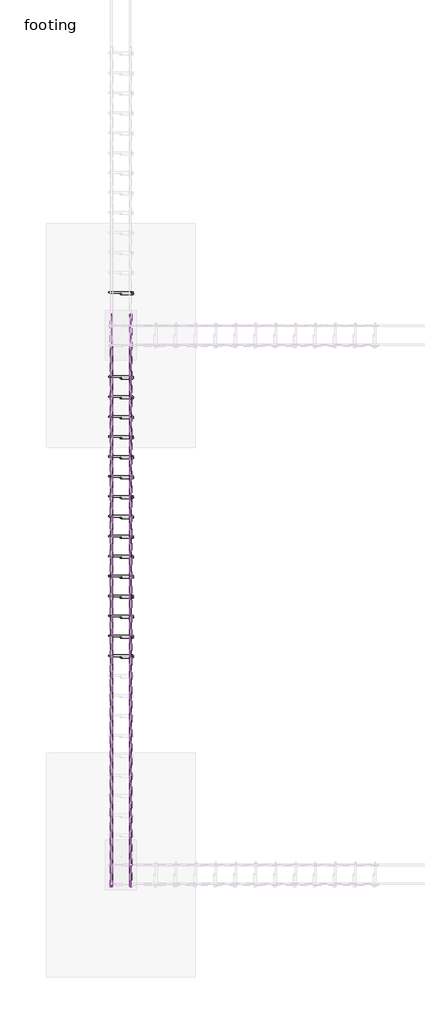
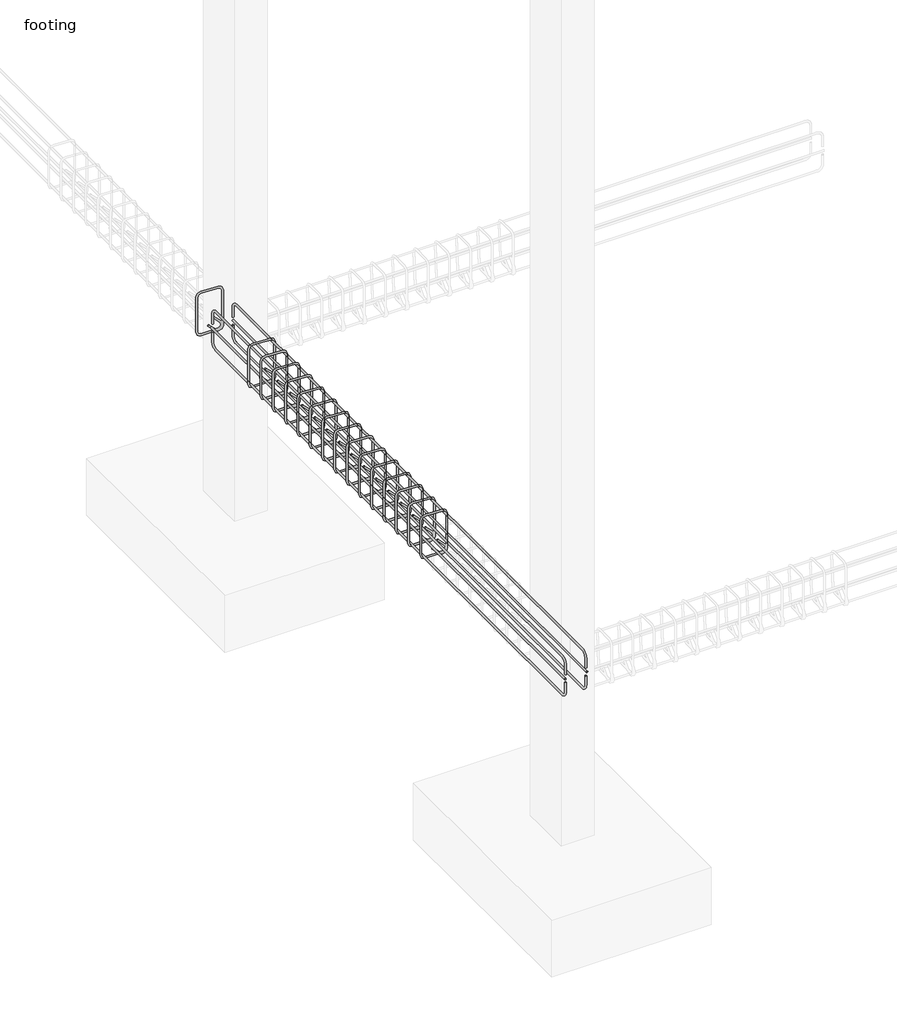
# One storey, part 4 of 21: 22 reinforcing bars.
"""IFC4 building model written with IfcOpenShell, lengths in millimetres."""

from ifc_helpers import new_model, si_unit, point, frame, origin, place, context, project, spatial, polyline, circle_curve, trimmed, segment, composite_curve, element, save
from ifc_brep_helpers import swept_disk

model = new_model("IFC4")

# Units and contexts
model_context = context("Model", 3, world=origin())
ifc_project = project(units=[si_unit("LENGTHUNIT", "METRE", prefix="MILLI")], contexts=[model_context])

# Site, building, storey
site = spatial("IfcSite", under=ifc_project)
building = spatial("IfcBuilding", under=site)
storey = spatial("IfcBuildingStorey", under=building, Name="footing", Elevation=-1524.0)

# Reinforcing bars
placement = place(None, origin())
element("IfcReinforcingBar", 1, at=placement, inside=storey, context=model_context, shape_type="SolidModel", body=[
    swept_disk(composite_curve([segment(polyline([(-12178.1165254, 1491.1956073, -265.9812362), (-12123.251527, 1491.1956073, -320.8462347)]), True, "CONTINUOUS"), segment(trimmed(circle_curve(frame((-12145.7021673, 1491.1956073, -343.296875), z_axis=(0.0, 1.0, 0.0), x_axis=(22.450640299999577, 0.0, 22.450640299999975)), 31.75), [point((-12123.251527, 1491.1956073, -320.8462347))], [point((-12145.7021673, 1491.1956073, -375.046875))], True, "CARTESIAN"), True, "CONTINUOUS"), segment(polyline([(-12145.7021673, 1491.1956073, -375.046875), (-12273.4959173, 1491.1956073, -375.046875)]), True, "CONTINUOUS"), segment(trimmed(circle_curve(frame((-12273.4959173, 1491.1956073, -343.296875), z_axis=(0.0, 1.0, 0.0), x_axis=(0.0, 0.0, -31.75)), 31.75), [point((-12273.4959173, 1491.1956073, -375.046875))], [point((-12305.2459173, 1491.1956073, -343.296875))], True, "CARTESIAN"), True, "CONTINUOUS"), segment(polyline([(-12305.2459173, 1491.1956073, -343.296875), (-12305.2459173, 1491.1956073, -63.103125)]), True, "CONTINUOUS"), segment(trimmed(circle_curve(frame((-12273.565658, 1489.0923536, -63.103125), z_axis=(0.0662442117686417, 0.9978034397651431, 0.0), x_axis=(-31.680259300001126, 2.1032536999998683, 0.0)), 31.75), [point((-12305.2459173, 1491.1956073, -63.103125))], [point((-12273.565658, 1489.0923536, -31.353125))], True, "CARTESIAN"), True, "CONTINUOUS"), segment(polyline([(-12273.565658, 1489.0923536, -31.353125), (-12145.6324265, 1480.598861, -31.353125)]), True, "CONTINUOUS"), segment(trimmed(circle_curve(frame((-12145.6324265, 1480.598861, -63.103125), z_axis=(0.06624421176864169, 0.997803439765143, 0.0), x_axis=(0.0, 0.0, 31.75)), 31.75), [point((-12145.6324265, 1480.598861, -31.353125))], [point((-12113.9521673, 1478.4956073, -63.103125))], True, "CARTESIAN"), True, "CONTINUOUS"), segment(polyline([(-12113.9521673, 1478.4956073, -63.103125), (-12113.9521673, 1478.4956073, -343.296875)]), True, "CONTINUOUS"), segment(trimmed(circle_curve(frame((-12145.7021673, 1478.4956073, -343.296875), z_axis=(0.0, 1.0, 0.0), x_axis=(31.75, 0.0, 0.0)), 31.75), [point((-12113.9521673, 1478.4956073, -343.296875))], [point((-12168.1528076, 1478.4956073, -365.7475153))], True, "CARTESIAN"), True, "CONTINUOUS"), segment(polyline([(-12168.1528076, 1478.4956073, -365.7475153), (-12223.017806, 1478.4956073, -310.8825168)]), True, "CONTINUOUS")], self_intersect=False), 6.35),
])
element("IfcReinforcingBar", 2, at=placement, inside=storey, context=model_context, shape_type="SolidModel", body=[
    swept_disk(composite_curve([segment(polyline([(-12178.1165254, 1653.8956073, -265.9812362), (-12123.251527, 1653.8956073, -320.8462347)]), True, "CONTINUOUS"), segment(trimmed(circle_curve(frame((-12145.7021673, 1653.8956073, -343.296875), z_axis=(0.0, 1.0, 0.0), x_axis=(22.450640299999577, 0.0, 22.450640299999975)), 31.75), [point((-12123.251527, 1653.8956073, -320.8462347))], [point((-12145.7021673, 1653.8956073, -375.046875))], True, "CARTESIAN"), True, "CONTINUOUS"), segment(polyline([(-12145.7021673, 1653.8956073, -375.046875), (-12273.4959173, 1653.8956073, -375.046875)]), True, "CONTINUOUS"), segment(trimmed(circle_curve(frame((-12273.4959173, 1653.8956073, -343.296875), z_axis=(0.0, 1.0, 0.0), x_axis=(0.0, 0.0, -31.75)), 31.75), [point((-12273.4959173, 1653.8956073, -375.046875))], [point((-12305.2459173, 1653.8956073, -343.296875))], True, "CARTESIAN"), True, "CONTINUOUS"), segment(polyline([(-12305.2459173, 1653.8956073, -343.296875), (-12305.2459173, 1653.8956073, -63.103125)]), True, "CONTINUOUS"), segment(trimmed(circle_curve(frame((-12273.565658, 1651.7923536, -63.103125), z_axis=(0.0662442117686417, 0.9978034397651431, 0.0), x_axis=(-31.680259300001126, 2.1032536999998683, 0.0)), 31.75), [point((-12305.2459173, 1653.8956073, -63.103125))], [point((-12273.565658, 1651.7923536, -31.353125))], True, "CARTESIAN"), True, "CONTINUOUS"), segment(polyline([(-12273.565658, 1651.7923536, -31.353125), (-12145.6324265, 1643.298861, -31.353125)]), True, "CONTINUOUS"), segment(trimmed(circle_curve(frame((-12145.6324265, 1643.298861, -63.103125), z_axis=(0.06624421176864169, 0.997803439765143, 0.0), x_axis=(0.0, 0.0, 31.75)), 31.75), [point((-12145.6324265, 1643.298861, -31.353125))], [point((-12113.9521673, 1641.1956073, -63.103125))], True, "CARTESIAN"), True, "CONTINUOUS"), segment(polyline([(-12113.9521673, 1641.1956073, -63.103125), (-12113.9521673, 1641.1956073, -343.296875)]), True, "CONTINUOUS"), segment(trimmed(circle_curve(frame((-12145.7021673, 1641.1956073, -343.296875), z_axis=(0.0, 1.0, 0.0), x_axis=(31.75, 0.0, 0.0)), 31.75), [point((-12113.9521673, 1641.1956073, -343.296875))], [point((-12168.1528076, 1641.1956073, -365.7475153))], True, "CARTESIAN"), True, "CONTINUOUS"), segment(polyline([(-12168.1528076, 1641.1956073, -365.7475153), (-12223.017806, 1641.1956073, -310.8825168)]), True, "CONTINUOUS")], self_intersect=False), 6.35),
])
element("IfcReinforcingBar", 3, at=placement, inside=storey, context=model_context, shape_type="SolidModel", body=[
    swept_disk(composite_curve([segment(polyline([(-12178.1165254, 1816.5956073, -265.9812362), (-12123.251527, 1816.5956073, -320.8462347)]), True, "CONTINUOUS"), segment(trimmed(circle_curve(frame((-12145.7021673, 1816.5956073, -343.296875), z_axis=(0.0, 1.0, 0.0), x_axis=(22.450640299999577, 0.0, 22.450640299999975)), 31.75), [point((-12123.251527, 1816.5956073, -320.8462347))], [point((-12145.7021673, 1816.5956073, -375.046875))], True, "CARTESIAN"), True, "CONTINUOUS"), segment(polyline([(-12145.7021673, 1816.5956073, -375.046875), (-12273.4959173, 1816.5956073, -375.046875)]), True, "CONTINUOUS"), segment(trimmed(circle_curve(frame((-12273.4959173, 1816.5956073, -343.296875), z_axis=(0.0, 1.0, 0.0), x_axis=(0.0, 0.0, -31.75)), 31.75), [point((-12273.4959173, 1816.5956073, -375.046875))], [point((-12305.2459173, 1816.5956073, -343.296875))], True, "CARTESIAN"), True, "CONTINUOUS"), segment(polyline([(-12305.2459173, 1816.5956073, -343.296875), (-12305.2459173, 1816.5956073, -63.103125)]), True, "CONTINUOUS"), segment(trimmed(circle_curve(frame((-12273.565658, 1814.4923536, -63.103125), z_axis=(0.0662442117686417, 0.9978034397651431, 0.0), x_axis=(-31.680259300001126, 2.1032537000000957, 0.0)), 31.75), [point((-12305.2459173, 1816.5956073, -63.103125))], [point((-12273.565658, 1814.4923536, -31.353125))], True, "CARTESIAN"), True, "CONTINUOUS"), segment(polyline([(-12273.565658, 1814.4923536, -31.353125), (-12145.6324265, 1805.998861, -31.353125)]), True, "CONTINUOUS"), segment(trimmed(circle_curve(frame((-12145.6324265, 1805.998861, -63.103125), z_axis=(0.06624421176864169, 0.997803439765143, 0.0), x_axis=(0.0, 0.0, 31.75)), 31.75), [point((-12145.6324265, 1805.998861, -31.353125))], [point((-12113.9521673, 1803.8956073, -63.103125))], True, "CARTESIAN"), True, "CONTINUOUS"), segment(polyline([(-12113.9521673, 1803.8956073, -63.103125), (-12113.9521673, 1803.8956073, -343.296875)]), True, "CONTINUOUS"), segment(trimmed(circle_curve(frame((-12145.7021673, 1803.8956073, -343.296875), z_axis=(0.0, 1.0, 0.0), x_axis=(31.75, 0.0, 0.0)), 31.75), [point((-12113.9521673, 1803.8956073, -343.296875))], [point((-12168.1528076, 1803.8956073, -365.7475153))], True, "CARTESIAN"), True, "CONTINUOUS"), segment(polyline([(-12168.1528076, 1803.8956073, -365.7475153), (-12223.017806, 1803.8956073, -310.8825168)]), True, "CONTINUOUS")], self_intersect=False), 6.35),
])
element("IfcReinforcingBar", 4, at=placement, inside=storey, context=model_context, shape_type="SolidModel", body=[
    swept_disk(composite_curve([segment(polyline([(-12178.1165254, 1979.2956073, -265.9812362), (-12123.251527, 1979.2956073, -320.8462347)]), True, "CONTINUOUS"), segment(trimmed(circle_curve(frame((-12145.7021673, 1979.2956073, -343.296875), z_axis=(0.0, 1.0, 0.0), x_axis=(22.450640299999577, 0.0, 22.450640299999975)), 31.75), [point((-12123.251527, 1979.2956073, -320.8462347))], [point((-12145.7021673, 1979.2956073, -375.046875))], True, "CARTESIAN"), True, "CONTINUOUS"), segment(polyline([(-12145.7021673, 1979.2956073, -375.046875), (-12273.4959173, 1979.2956073, -375.046875)]), True, "CONTINUOUS"), segment(trimmed(circle_curve(frame((-12273.4959173, 1979.2956073, -343.296875), z_axis=(0.0, 1.0, 0.0), x_axis=(0.0, 0.0, -31.75)), 31.75), [point((-12273.4959173, 1979.2956073, -375.046875))], [point((-12305.2459173, 1979.2956073, -343.296875))], True, "CARTESIAN"), True, "CONTINUOUS"), segment(polyline([(-12305.2459173, 1979.2956073, -343.296875), (-12305.2459173, 1979.2956073, -63.103125)]), True, "CONTINUOUS"), segment(trimmed(circle_curve(frame((-12273.565658, 1977.1923536, -63.103125), z_axis=(0.0662442117686417, 0.9978034397651431, 0.0), x_axis=(-31.680259300001126, 2.1032537000000957, 0.0)), 31.75), [point((-12305.2459173, 1979.2956073, -63.103125))], [point((-12273.565658, 1977.1923536, -31.353125))], True, "CARTESIAN"), True, "CONTINUOUS"), segment(polyline([(-12273.565658, 1977.1923536, -31.353125), (-12145.6324265, 1968.698861, -31.353125)]), True, "CONTINUOUS"), segment(trimmed(circle_curve(frame((-12145.6324265, 1968.698861, -63.103125), z_axis=(0.06624421176864169, 0.997803439765143, 0.0), x_axis=(0.0, 0.0, 31.75)), 31.75), [point((-12145.6324265, 1968.698861, -31.353125))], [point((-12113.9521673, 1966.5956073, -63.103125))], True, "CARTESIAN"), True, "CONTINUOUS"), segment(polyline([(-12113.9521673, 1966.5956073, -63.103125), (-12113.9521673, 1966.5956073, -343.296875)]), True, "CONTINUOUS"), segment(trimmed(circle_curve(frame((-12145.7021673, 1966.5956073, -343.296875), z_axis=(0.0, 1.0, 0.0), x_axis=(31.75, 0.0, 0.0)), 31.75), [point((-12113.9521673, 1966.5956073, -343.296875))], [point((-12168.1528076, 1966.5956073, -365.7475153))], True, "CARTESIAN"), True, "CONTINUOUS"), segment(polyline([(-12168.1528076, 1966.5956073, -365.7475153), (-12223.017806, 1966.5956073, -310.8825168)]), True, "CONTINUOUS")], self_intersect=False), 6.35),
])
element("IfcReinforcingBar", 5, at=placement, inside=storey, context=model_context, shape_type="SolidModel", body=[
    swept_disk(composite_curve([segment(polyline([(-12178.1165254, 2141.9956073, -265.9812362), (-12123.251527, 2141.9956073, -320.8462347)]), True, "CONTINUOUS"), segment(trimmed(circle_curve(frame((-12145.7021673, 2141.9956073, -343.296875), z_axis=(0.0, 1.0, 0.0), x_axis=(22.450640299999577, 0.0, 22.450640299999975)), 31.75), [point((-12123.251527, 2141.9956073, -320.8462347))], [point((-12145.7021673, 2141.9956073, -375.046875))], True, "CARTESIAN"), True, "CONTINUOUS"), segment(polyline([(-12145.7021673, 2141.9956073, -375.046875), (-12273.4959173, 2141.9956073, -375.046875)]), True, "CONTINUOUS"), segment(trimmed(circle_curve(frame((-12273.4959173, 2141.9956073, -343.296875), z_axis=(0.0, 1.0, 0.0), x_axis=(0.0, 0.0, -31.75)), 31.75), [point((-12273.4959173, 2141.9956073, -375.046875))], [point((-12305.2459173, 2141.9956073, -343.296875))], True, "CARTESIAN"), True, "CONTINUOUS"), segment(polyline([(-12305.2459173, 2141.9956073, -343.296875), (-12305.2459173, 2141.9956073, -63.103125)]), True, "CONTINUOUS"), segment(trimmed(circle_curve(frame((-12273.565658, 2139.8923536, -63.103125), z_axis=(0.0662442117686417, 0.9978034397651431, 0.0), x_axis=(-31.680259300001126, 2.103253699999641, 0.0)), 31.75), [point((-12305.2459173, 2141.9956073, -63.103125))], [point((-12273.565658, 2139.8923536, -31.353125))], True, "CARTESIAN"), True, "CONTINUOUS"), segment(polyline([(-12273.565658, 2139.8923536, -31.353125), (-12145.6324265, 2131.398861, -31.353125)]), True, "CONTINUOUS"), segment(trimmed(circle_curve(frame((-12145.6324265, 2131.398861, -63.103125), z_axis=(0.06624421176864169, 0.997803439765143, 0.0), x_axis=(0.0, 0.0, 31.75)), 31.75), [point((-12145.6324265, 2131.398861, -31.353125))], [point((-12113.9521673, 2129.2956073, -63.103125))], True, "CARTESIAN"), True, "CONTINUOUS"), segment(polyline([(-12113.9521673, 2129.2956073, -63.103125), (-12113.9521673, 2129.2956073, -343.296875)]), True, "CONTINUOUS"), segment(trimmed(circle_curve(frame((-12145.7021673, 2129.2956073, -343.296875), z_axis=(0.0, 1.0, 0.0), x_axis=(31.75, 0.0, 0.0)), 31.75), [point((-12113.9521673, 2129.2956073, -343.296875))], [point((-12168.1528076, 2129.2956073, -365.7475153))], True, "CARTESIAN"), True, "CONTINUOUS"), segment(polyline([(-12168.1528076, 2129.2956073, -365.7475153), (-12223.017806, 2129.2956073, -310.8825168)]), True, "CONTINUOUS")], self_intersect=False), 6.35),
])
element("IfcReinforcingBar", 6, at=placement, inside=storey, context=model_context, shape_type="SolidModel", body=[
    swept_disk(composite_curve([segment(polyline([(-12178.1165254, 2304.6956073, -265.9812362), (-12123.251527, 2304.6956073, -320.8462347)]), True, "CONTINUOUS"), segment(trimmed(circle_curve(frame((-12145.7021673, 2304.6956073, -343.296875), z_axis=(0.0, 1.0, 0.0), x_axis=(22.450640299999577, 0.0, 22.450640299999975)), 31.75), [point((-12123.251527, 2304.6956073, -320.8462347))], [point((-12145.7021673, 2304.6956073, -375.046875))], True, "CARTESIAN"), True, "CONTINUOUS"), segment(polyline([(-12145.7021673, 2304.6956073, -375.046875), (-12273.4959173, 2304.6956073, -375.046875)]), True, "CONTINUOUS"), segment(trimmed(circle_curve(frame((-12273.4959173, 2304.6956073, -343.296875), z_axis=(0.0, 1.0, 0.0), x_axis=(0.0, 0.0, -31.75)), 31.75), [point((-12273.4959173, 2304.6956073, -375.046875))], [point((-12305.2459173, 2304.6956073, -343.296875))], True, "CARTESIAN"), True, "CONTINUOUS"), segment(polyline([(-12305.2459173, 2304.6956073, -343.296875), (-12305.2459173, 2304.6956073, -63.103125)]), True, "CONTINUOUS"), segment(trimmed(circle_curve(frame((-12273.565658, 2302.5923536, -63.103125), z_axis=(0.0662442117686417, 0.9978034397651431, 0.0), x_axis=(-31.680259300001126, 2.1032537000000957, 0.0)), 31.75), [point((-12305.2459173, 2304.6956073, -63.103125))], [point((-12273.565658, 2302.5923536, -31.353125))], True, "CARTESIAN"), True, "CONTINUOUS"), segment(polyline([(-12273.565658, 2302.5923536, -31.353125), (-12145.6324265, 2294.098861, -31.353125)]), True, "CONTINUOUS"), segment(trimmed(circle_curve(frame((-12145.6324265, 2294.098861, -63.103125), z_axis=(0.06624421176864169, 0.997803439765143, 0.0), x_axis=(0.0, 0.0, 31.75)), 31.75), [point((-12145.6324265, 2294.098861, -31.353125))], [point((-12113.9521673, 2291.9956073, -63.103125))], True, "CARTESIAN"), True, "CONTINUOUS"), segment(polyline([(-12113.9521673, 2291.9956073, -63.103125), (-12113.9521673, 2291.9956073, -343.296875)]), True, "CONTINUOUS"), segment(trimmed(circle_curve(frame((-12145.7021673, 2291.9956073, -343.296875), z_axis=(0.0, 1.0, 0.0), x_axis=(31.75, 0.0, 0.0)), 31.75), [point((-12113.9521673, 2291.9956073, -343.296875))], [point((-12168.1528076, 2291.9956073, -365.7475153))], True, "CARTESIAN"), True, "CONTINUOUS"), segment(polyline([(-12168.1528076, 2291.9956073, -365.7475153), (-12223.017806, 2291.9956073, -310.8825168)]), True, "CONTINUOUS")], self_intersect=False), 6.35),
])
element("IfcReinforcingBar", 7, at=placement, inside=storey, context=model_context, shape_type="SolidModel", body=[
    swept_disk(composite_curve([segment(polyline([(-12178.1165254, 2467.3956073, -265.9812362), (-12123.251527, 2467.3956073, -320.8462347)]), True, "CONTINUOUS"), segment(trimmed(circle_curve(frame((-12145.7021673, 2467.3956073, -343.296875), z_axis=(0.0, 1.0, 0.0), x_axis=(22.450640299999577, 0.0, 22.450640299999975)), 31.75), [point((-12123.251527, 2467.3956073, -320.8462347))], [point((-12145.7021673, 2467.3956073, -375.046875))], True, "CARTESIAN"), True, "CONTINUOUS"), segment(polyline([(-12145.7021673, 2467.3956073, -375.046875), (-12273.4959173, 2467.3956073, -375.046875)]), True, "CONTINUOUS"), segment(trimmed(circle_curve(frame((-12273.4959173, 2467.3956073, -343.296875), z_axis=(0.0, 1.0, 0.0), x_axis=(0.0, 0.0, -31.75)), 31.75), [point((-12273.4959173, 2467.3956073, -375.046875))], [point((-12305.2459173, 2467.3956073, -343.296875))], True, "CARTESIAN"), True, "CONTINUOUS"), segment(polyline([(-12305.2459173, 2467.3956073, -343.296875), (-12305.2459173, 2467.3956073, -63.103125)]), True, "CONTINUOUS"), segment(trimmed(circle_curve(frame((-12273.565658, 2465.2923536, -63.103125), z_axis=(0.0662442117686417, 0.9978034397651431, 0.0), x_axis=(-31.680259300001126, 2.1032537000000957, 0.0)), 31.75), [point((-12305.2459173, 2467.3956073, -63.103125))], [point((-12273.565658, 2465.2923536, -31.353125))], True, "CARTESIAN"), True, "CONTINUOUS"), segment(polyline([(-12273.565658, 2465.2923536, -31.353125), (-12145.6324265, 2456.798861, -31.353125)]), True, "CONTINUOUS"), segment(trimmed(circle_curve(frame((-12145.6324265, 2456.798861, -63.103125), z_axis=(0.06624421176864169, 0.997803439765143, 0.0), x_axis=(0.0, 0.0, 31.75)), 31.75), [point((-12145.6324265, 2456.798861, -31.353125))], [point((-12113.9521673, 2454.6956073, -63.103125))], True, "CARTESIAN"), True, "CONTINUOUS"), segment(polyline([(-12113.9521673, 2454.6956073, -63.103125), (-12113.9521673, 2454.6956073, -343.296875)]), True, "CONTINUOUS"), segment(trimmed(circle_curve(frame((-12145.7021673, 2454.6956073, -343.296875), z_axis=(0.0, 1.0, 0.0), x_axis=(31.75, 0.0, 0.0)), 31.75), [point((-12113.9521673, 2454.6956073, -343.296875))], [point((-12168.1528076, 2454.6956073, -365.7475153))], True, "CARTESIAN"), True, "CONTINUOUS"), segment(polyline([(-12168.1528076, 2454.6956073, -365.7475153), (-12223.017806, 2454.6956073, -310.8825168)]), True, "CONTINUOUS")], self_intersect=False), 6.35),
])
element("IfcReinforcingBar", 8, at=placement, inside=storey, context=model_context, shape_type="SolidModel", body=[
    swept_disk(composite_curve([segment(polyline([(-12178.1165254, 2630.0956073, -265.9812362), (-12123.251527, 2630.0956073, -320.8462347)]), True, "CONTINUOUS"), segment(trimmed(circle_curve(frame((-12145.7021673, 2630.0956073, -343.296875), z_axis=(0.0, 1.0, 0.0), x_axis=(22.450640299999577, 0.0, 22.450640299999975)), 31.75), [point((-12123.251527, 2630.0956073, -320.8462347))], [point((-12145.7021673, 2630.0956073, -375.046875))], True, "CARTESIAN"), True, "CONTINUOUS"), segment(polyline([(-12145.7021673, 2630.0956073, -375.046875), (-12273.4959173, 2630.0956073, -375.046875)]), True, "CONTINUOUS"), segment(trimmed(circle_curve(frame((-12273.4959173, 2630.0956073, -343.296875), z_axis=(0.0, 1.0, 0.0), x_axis=(0.0, 0.0, -31.75)), 31.75), [point((-12273.4959173, 2630.0956073, -375.046875))], [point((-12305.2459173, 2630.0956073, -343.296875))], True, "CARTESIAN"), True, "CONTINUOUS"), segment(polyline([(-12305.2459173, 2630.0956073, -343.296875), (-12305.2459173, 2630.0956073, -63.103125)]), True, "CONTINUOUS"), segment(trimmed(circle_curve(frame((-12273.565658, 2627.9923536, -63.103125), z_axis=(0.0662442117686417, 0.9978034397651431, 0.0), x_axis=(-31.680259300001126, 2.1032537000000957, 0.0)), 31.75), [point((-12305.2459173, 2630.0956073, -63.103125))], [point((-12273.565658, 2627.9923536, -31.353125))], True, "CARTESIAN"), True, "CONTINUOUS"), segment(polyline([(-12273.565658, 2627.9923536, -31.353125), (-12145.6324265, 2619.498861, -31.353125)]), True, "CONTINUOUS"), segment(trimmed(circle_curve(frame((-12145.6324265, 2619.498861, -63.103125), z_axis=(0.06624421176864169, 0.997803439765143, 0.0), x_axis=(0.0, 0.0, 31.75)), 31.75), [point((-12145.6324265, 2619.498861, -31.353125))], [point((-12113.9521673, 2617.3956073, -63.103125))], True, "CARTESIAN"), True, "CONTINUOUS"), segment(polyline([(-12113.9521673, 2617.3956073, -63.103125), (-12113.9521673, 2617.3956073, -343.296875)]), True, "CONTINUOUS"), segment(trimmed(circle_curve(frame((-12145.7021673, 2617.3956073, -343.296875), z_axis=(0.0, 1.0, 0.0), x_axis=(31.75, 0.0, 0.0)), 31.75), [point((-12113.9521673, 2617.3956073, -343.296875))], [point((-12168.1528076, 2617.3956073, -365.7475153))], True, "CARTESIAN"), True, "CONTINUOUS"), segment(polyline([(-12168.1528076, 2617.3956073, -365.7475153), (-12223.017806, 2617.3956073, -310.8825168)]), True, "CONTINUOUS")], self_intersect=False), 6.35),
])
element("IfcReinforcingBar", 9, at=placement, inside=storey, context=model_context, shape_type="SolidModel", body=[
    swept_disk(composite_curve([segment(polyline([(-12178.1165254, 2792.7956073, -265.9812362), (-12123.251527, 2792.7956073, -320.8462347)]), True, "CONTINUOUS"), segment(trimmed(circle_curve(frame((-12145.7021673, 2792.7956073, -343.296875), z_axis=(0.0, 1.0, 0.0), x_axis=(22.450640299999577, 0.0, 22.450640299999975)), 31.75), [point((-12123.251527, 2792.7956073, -320.8462347))], [point((-12145.7021673, 2792.7956073, -375.046875))], True, "CARTESIAN"), True, "CONTINUOUS"), segment(polyline([(-12145.7021673, 2792.7956073, -375.046875), (-12273.4959173, 2792.7956073, -375.046875)]), True, "CONTINUOUS"), segment(trimmed(circle_curve(frame((-12273.4959173, 2792.7956073, -343.296875), z_axis=(0.0, 1.0, 0.0), x_axis=(0.0, 0.0, -31.75)), 31.75), [point((-12273.4959173, 2792.7956073, -375.046875))], [point((-12305.2459173, 2792.7956073, -343.296875))], True, "CARTESIAN"), True, "CONTINUOUS"), segment(polyline([(-12305.2459173, 2792.7956073, -343.296875), (-12305.2459173, 2792.7956073, -63.103125)]), True, "CONTINUOUS"), segment(trimmed(circle_curve(frame((-12273.565658, 2790.6923536, -63.103125), z_axis=(0.0662442117686417, 0.9978034397651431, 0.0), x_axis=(-31.680259300001126, 2.1032537000000957, 0.0)), 31.75), [point((-12305.2459173, 2792.7956073, -63.103125))], [point((-12273.565658, 2790.6923536, -31.353125))], True, "CARTESIAN"), True, "CONTINUOUS"), segment(polyline([(-12273.565658, 2790.6923536, -31.353125), (-12145.6324265, 2782.198861, -31.353125)]), True, "CONTINUOUS"), segment(trimmed(circle_curve(frame((-12145.6324265, 2782.198861, -63.103125), z_axis=(0.06624421176864169, 0.997803439765143, 0.0), x_axis=(0.0, 0.0, 31.75)), 31.75), [point((-12145.6324265, 2782.198861, -31.353125))], [point((-12113.9521673, 2780.0956073, -63.103125))], True, "CARTESIAN"), True, "CONTINUOUS"), segment(polyline([(-12113.9521673, 2780.0956073, -63.103125), (-12113.9521673, 2780.0956073, -343.296875)]), True, "CONTINUOUS"), segment(trimmed(circle_curve(frame((-12145.7021673, 2780.0956073, -343.296875), z_axis=(0.0, 1.0, 0.0), x_axis=(31.75, 0.0, 0.0)), 31.75), [point((-12113.9521673, 2780.0956073, -343.296875))], [point((-12168.1528076, 2780.0956073, -365.7475153))], True, "CARTESIAN"), True, "CONTINUOUS"), segment(polyline([(-12168.1528076, 2780.0956073, -365.7475153), (-12223.017806, 2780.0956073, -310.8825168)]), True, "CONTINUOUS")], self_intersect=False), 6.35),
])
element("IfcReinforcingBar", 10, at=placement, inside=storey, context=model_context, shape_type="SolidModel", body=[
    swept_disk(composite_curve([segment(polyline([(-12178.1165254, 2955.4956073, -265.9812362), (-12123.251527, 2955.4956073, -320.8462347)]), True, "CONTINUOUS"), segment(trimmed(circle_curve(frame((-12145.7021673, 2955.4956073, -343.296875), z_axis=(0.0, 1.0, 0.0), x_axis=(22.450640299999577, 0.0, 22.450640299999975)), 31.75), [point((-12123.251527, 2955.4956073, -320.8462347))], [point((-12145.7021673, 2955.4956073, -375.046875))], True, "CARTESIAN"), True, "CONTINUOUS"), segment(polyline([(-12145.7021673, 2955.4956073, -375.046875), (-12273.4959173, 2955.4956073, -375.046875)]), True, "CONTINUOUS"), segment(trimmed(circle_curve(frame((-12273.4959173, 2955.4956073, -343.296875), z_axis=(0.0, 1.0, 0.0), x_axis=(0.0, 0.0, -31.75)), 31.75), [point((-12273.4959173, 2955.4956073, -375.046875))], [point((-12305.2459173, 2955.4956073, -343.296875))], True, "CARTESIAN"), True, "CONTINUOUS"), segment(polyline([(-12305.2459173, 2955.4956073, -343.296875), (-12305.2459173, 2955.4956073, -63.103125)]), True, "CONTINUOUS"), segment(trimmed(circle_curve(frame((-12273.565658, 2953.3923536, -63.103125), z_axis=(0.0662442117686417, 0.9978034397651431, 0.0), x_axis=(-31.680259300001126, 2.103253699999641, 0.0)), 31.75), [point((-12305.2459173, 2955.4956073, -63.103125))], [point((-12273.565658, 2953.3923536, -31.353125))], True, "CARTESIAN"), True, "CONTINUOUS"), segment(polyline([(-12273.565658, 2953.3923536, -31.353125), (-12145.6324265, 2944.898861, -31.353125)]), True, "CONTINUOUS"), segment(trimmed(circle_curve(frame((-12145.6324265, 2944.898861, -63.103125), z_axis=(0.06624421176864169, 0.997803439765143, 0.0), x_axis=(0.0, 0.0, 31.75)), 31.75), [point((-12145.6324265, 2944.898861, -31.353125))], [point((-12113.9521673, 2942.7956073, -63.103125))], True, "CARTESIAN"), True, "CONTINUOUS"), segment(polyline([(-12113.9521673, 2942.7956073, -63.103125), (-12113.9521673, 2942.7956073, -343.296875)]), True, "CONTINUOUS"), segment(trimmed(circle_curve(frame((-12145.7021673, 2942.7956073, -343.296875), z_axis=(0.0, 1.0, 0.0), x_axis=(31.75, 0.0, 0.0)), 31.75), [point((-12113.9521673, 2942.7956073, -343.296875))], [point((-12168.1528076, 2942.7956073, -365.7475153))], True, "CARTESIAN"), True, "CONTINUOUS"), segment(polyline([(-12168.1528076, 2942.7956073, -365.7475153), (-12223.017806, 2942.7956073, -310.8825168)]), True, "CONTINUOUS")], self_intersect=False), 6.35),
])
element("IfcReinforcingBar", 11, at=placement, inside=storey, context=model_context, shape_type="SolidModel", body=[
    swept_disk(composite_curve([segment(polyline([(-12178.1165254, 3118.1956073, -265.9812362), (-12123.251527, 3118.1956073, -320.8462347)]), True, "CONTINUOUS"), segment(trimmed(circle_curve(frame((-12145.7021673, 3118.1956073, -343.296875), z_axis=(0.0, 1.0, 0.0), x_axis=(22.450640299999577, 0.0, 22.450640299999975)), 31.75), [point((-12123.251527, 3118.1956073, -320.8462347))], [point((-12145.7021673, 3118.1956073, -375.046875))], True, "CARTESIAN"), True, "CONTINUOUS"), segment(polyline([(-12145.7021673, 3118.1956073, -375.046875), (-12273.4959173, 3118.1956073, -375.046875)]), True, "CONTINUOUS"), segment(trimmed(circle_curve(frame((-12273.4959173, 3118.1956073, -343.296875), z_axis=(0.0, 1.0, 0.0), x_axis=(0.0, 0.0, -31.75)), 31.75), [point((-12273.4959173, 3118.1956073, -375.046875))], [point((-12305.2459173, 3118.1956073, -343.296875))], True, "CARTESIAN"), True, "CONTINUOUS"), segment(polyline([(-12305.2459173, 3118.1956073, -343.296875), (-12305.2459173, 3118.1956073, -63.103125)]), True, "CONTINUOUS"), segment(trimmed(circle_curve(frame((-12273.565658, 3116.0923536, -63.103125), z_axis=(0.0662442117686417, 0.9978034397651431, 0.0), x_axis=(-31.680259300001126, 2.1032537000000957, 0.0)), 31.75), [point((-12305.2459173, 3118.1956073, -63.103125))], [point((-12273.565658, 3116.0923536, -31.353125))], True, "CARTESIAN"), True, "CONTINUOUS"), segment(polyline([(-12273.565658, 3116.0923536, -31.353125), (-12145.6324265, 3107.598861, -31.353125)]), True, "CONTINUOUS"), segment(trimmed(circle_curve(frame((-12145.6324265, 3107.598861, -63.103125), z_axis=(0.06624421176864169, 0.997803439765143, 0.0), x_axis=(0.0, 0.0, 31.75)), 31.75), [point((-12145.6324265, 3107.598861, -31.353125))], [point((-12113.9521673, 3105.4956073, -63.103125))], True, "CARTESIAN"), True, "CONTINUOUS"), segment(polyline([(-12113.9521673, 3105.4956073, -63.103125), (-12113.9521673, 3105.4956073, -343.296875)]), True, "CONTINUOUS"), segment(trimmed(circle_curve(frame((-12145.7021673, 3105.4956073, -343.296875), z_axis=(0.0, 1.0, 0.0), x_axis=(31.75, 0.0, 0.0)), 31.75), [point((-12113.9521673, 3105.4956073, -343.296875))], [point((-12168.1528076, 3105.4956073, -365.7475153))], True, "CARTESIAN"), True, "CONTINUOUS"), segment(polyline([(-12168.1528076, 3105.4956073, -365.7475153), (-12223.017806, 3105.4956073, -310.8825168)]), True, "CONTINUOUS")], self_intersect=False), 6.35),
])
element("IfcReinforcingBar", 12, at=placement, inside=storey, context=model_context, shape_type="SolidModel", body=[
    swept_disk(composite_curve([segment(polyline([(-12178.1165254, 3280.8956073, -265.9812362), (-12123.251527, 3280.8956073, -320.8462347)]), True, "CONTINUOUS"), segment(trimmed(circle_curve(frame((-12145.7021673, 3280.8956073, -343.296875), z_axis=(0.0, 1.0, 0.0), x_axis=(22.450640299999577, 0.0, 22.450640299999975)), 31.75), [point((-12123.251527, 3280.8956073, -320.8462347))], [point((-12145.7021673, 3280.8956073, -375.046875))], True, "CARTESIAN"), True, "CONTINUOUS"), segment(polyline([(-12145.7021673, 3280.8956073, -375.046875), (-12273.4959173, 3280.8956073, -375.046875)]), True, "CONTINUOUS"), segment(trimmed(circle_curve(frame((-12273.4959173, 3280.8956073, -343.296875), z_axis=(0.0, 1.0, 0.0), x_axis=(0.0, 0.0, -31.75)), 31.75), [point((-12273.4959173, 3280.8956073, -375.046875))], [point((-12305.2459173, 3280.8956073, -343.296875))], True, "CARTESIAN"), True, "CONTINUOUS"), segment(polyline([(-12305.2459173, 3280.8956073, -343.296875), (-12305.2459173, 3280.8956073, -63.103125)]), True, "CONTINUOUS"), segment(trimmed(circle_curve(frame((-12273.565658, 3278.7923536, -63.103125), z_axis=(0.0662442117686417, 0.9978034397651431, 0.0), x_axis=(-31.680259300001126, 2.1032537000000957, 0.0)), 31.75), [point((-12305.2459173, 3280.8956073, -63.103125))], [point((-12273.565658, 3278.7923536, -31.353125))], True, "CARTESIAN"), True, "CONTINUOUS"), segment(polyline([(-12273.565658, 3278.7923536, -31.353125), (-12145.6324265, 3270.298861, -31.353125)]), True, "CONTINUOUS"), segment(trimmed(circle_curve(frame((-12145.6324265, 3270.298861, -63.103125), z_axis=(0.06624421176864169, 0.997803439765143, 0.0), x_axis=(0.0, 0.0, 31.75)), 31.75), [point((-12145.6324265, 3270.298861, -31.353125))], [point((-12113.9521673, 3268.1956073, -63.103125))], True, "CARTESIAN"), True, "CONTINUOUS"), segment(polyline([(-12113.9521673, 3268.1956073, -63.103125), (-12113.9521673, 3268.1956073, -343.296875)]), True, "CONTINUOUS"), segment(trimmed(circle_curve(frame((-12145.7021673, 3268.1956073, -343.296875), z_axis=(0.0, 1.0, 0.0), x_axis=(31.75, 0.0, 0.0)), 31.75), [point((-12113.9521673, 3268.1956073, -343.296875))], [point((-12168.1528076, 3268.1956073, -365.7475153))], True, "CARTESIAN"), True, "CONTINUOUS"), segment(polyline([(-12168.1528076, 3268.1956073, -365.7475153), (-12223.017806, 3268.1956073, -310.8825168)]), True, "CONTINUOUS")], self_intersect=False), 6.35),
])
element("IfcReinforcingBar", 13, at=placement, inside=storey, context=model_context, shape_type="SolidModel", body=[
    swept_disk(composite_curve([segment(polyline([(-12132.2317831, -391.7269256, -170.2827408), (-12132.2317831, -391.7269256, -94.0827408)]), True, "CONTINUOUS"), segment(trimmed(circle_curve(frame((-12132.2317831, -347.2769256, -94.0827408), z_axis=(-1.0, 0.0, 0.0), x_axis=(0.0, -44.44999999999999, 0.0)), 44.45), [point((-12132.2317831, -391.7269256, -94.0827408))], [point((-12132.2317831, -347.2769256, -49.6327408))], True, "CARTESIAN"), True, "CONTINUOUS"), segment(polyline([(-12132.2317831, -347.2769256, -49.6327408), (-12132.2317831, 4231.8668244, -49.6327408)]), True, "CONTINUOUS"), segment(trimmed(circle_curve(frame((-12132.2317831, 4231.8668244, -94.0827408), z_axis=(-1.0, 0.0, 0.0), x_axis=(0.0, 0.0, 44.449999999999996)), 44.45), [point((-12132.2317831, 4231.8668244, -49.6327408))], [point((-12132.2317831, 4276.3168244, -94.0827408))], True, "CARTESIAN"), True, "CONTINUOUS"), segment(polyline([(-12132.2317831, 4276.3168244, -94.0827408), (-12132.2317831, 4276.3168244, -170.2827408)]), True, "CONTINUOUS")], self_intersect=False), 6.35),
])
element("IfcReinforcingBar", 14, at=placement, inside=storey, context=model_context, shape_type="SolidModel", body=[
    swept_disk(composite_curve([segment(polyline([(-12286.9663014, -391.7269256, -170.2827408), (-12286.9663014, -391.7269256, -94.0827408)]), True, "CONTINUOUS"), segment(trimmed(circle_curve(frame((-12286.9663014, -347.2769256, -94.0827408), z_axis=(-1.0, 0.0, 0.0), x_axis=(0.0, -44.44999999999999, 0.0)), 44.45), [point((-12286.9663014, -391.7269256, -94.0827408))], [point((-12286.9663014, -347.2769256, -49.6327408))], True, "CARTESIAN"), True, "CONTINUOUS"), segment(polyline([(-12286.9663014, -347.2769256, -49.6327408), (-12286.9663014, 4231.8668244, -49.6327408)]), True, "CONTINUOUS"), segment(trimmed(circle_curve(frame((-12286.9663014, 4231.8668244, -94.0827408), z_axis=(-1.0, 0.0, 0.0), x_axis=(0.0, 0.0, 44.449999999999996)), 44.45), [point((-12286.9663014, 4231.8668244, -49.6327408))], [point((-12286.9663014, 4276.3168244, -94.0827408))], True, "CARTESIAN"), True, "CONTINUOUS"), segment(polyline([(-12286.9663014, 4276.3168244, -94.0827408), (-12286.9663014, 4276.3168244, -170.2827408)]), True, "CONTINUOUS")], self_intersect=False), 6.35),
])
element("IfcReinforcingBar", 15, at=placement, inside=storey, context=model_context, shape_type="SolidModel", body=[
    swept_disk(composite_curve([segment(polyline([(-12132.2317831, -391.7269256, -236.1172592), (-12132.2317831, -391.7269256, -312.3172592)]), True, "CONTINUOUS"), segment(trimmed(circle_curve(frame((-12132.2317831, -347.2769256, -312.3172592), z_axis=(1.0, 0.0, 0.0), x_axis=(0.0, -44.44999999999999, 0.0)), 44.45), [point((-12132.2317831, -391.7269256, -312.3172592))], [point((-12132.2317831, -347.2769256, -356.7672592))], True, "CARTESIAN"), True, "CONTINUOUS"), segment(polyline([(-12132.2317831, -347.2769256, -356.7672592), (-12132.2317831, 4231.8668244, -356.7672592)]), True, "CONTINUOUS"), segment(trimmed(circle_curve(frame((-12132.2317831, 4231.8668244, -312.3172592), z_axis=(1.0, 0.0, 0.0), x_axis=(0.0, 0.0, -44.44999999999999)), 44.45), [point((-12132.2317831, 4231.8668244, -356.7672592))], [point((-12132.2317831, 4276.3168244, -312.3172592))], True, "CARTESIAN"), True, "CONTINUOUS"), segment(polyline([(-12132.2317831, 4276.3168244, -312.3172592), (-12132.2317831, 4276.3168244, -236.1172592)]), True, "CONTINUOUS")], self_intersect=False), 6.35),
])
element("IfcReinforcingBar", 16, at=placement, inside=storey, context=model_context, shape_type="SolidModel", body=[
    swept_disk(composite_curve([segment(polyline([(-12286.9663014, -391.7269256, -236.1172592), (-12286.9663014, -391.7269256, -312.3172592)]), True, "CONTINUOUS"), segment(trimmed(circle_curve(frame((-12286.9663014, -347.2769256, -312.3172592), z_axis=(1.0, 0.0, 0.0), x_axis=(0.0, -44.44999999999999, 0.0)), 44.45), [point((-12286.9663014, -391.7269256, -312.3172592))], [point((-12286.9663014, -347.2769256, -356.7672592))], True, "CARTESIAN"), True, "CONTINUOUS"), segment(polyline([(-12286.9663014, -347.2769256, -356.7672592), (-12286.9663014, 4231.8668244, -356.7672592)]), True, "CONTINUOUS"), segment(trimmed(circle_curve(frame((-12286.9663014, 4231.8668244, -312.3172592), z_axis=(1.0, 0.0, 0.0), x_axis=(0.0, 0.0, -44.44999999999999)), 44.45), [point((-12286.9663014, 4231.8668244, -356.7672592))], [point((-12286.9663014, 4276.3168244, -312.3172592))], True, "CARTESIAN"), True, "CONTINUOUS"), segment(polyline([(-12286.9663014, 4276.3168244, -312.3172592), (-12286.9663014, 4276.3168244, -236.1172592)]), True, "CONTINUOUS")], self_intersect=False), 6.35),
])
element("IfcReinforcingBar", 17, at=placement, inside=storey, context=model_context, shape_type="SolidModel", body=[
    swept_disk(composite_curve([segment(polyline([(-12126.6521673, -398.0769256, -203.2), (-12126.6521673, 4282.6668244, -203.2)]), True, "CONTINUOUS")], self_intersect=False), 6.35),
])
element("IfcReinforcingBar", 18, at=placement, inside=storey, context=model_context, shape_type="SolidModel", body=[
    swept_disk(composite_curve([segment(polyline([(-12292.5459173, -398.0769256, -203.2), (-12292.5459173, 4282.6668244, -203.2)]), True, "CONTINUOUS")], self_intersect=False), 6.35),
])
element("IfcReinforcingBar", 19, at=placement, inside=storey, context=model_context, shape_type="SolidModel", body=[
    swept_disk(composite_curve([segment(polyline([(-12178.1165254, 3443.5956073, -265.9812362), (-12123.251527, 3443.5956073, -320.8462347)]), True, "CONTINUOUS"), segment(trimmed(circle_curve(frame((-12145.7021673, 3443.5956073, -343.296875), z_axis=(0.0, 1.0, 0.0), x_axis=(22.450640299999577, 0.0, 22.450640299999975)), 31.75), [point((-12123.251527, 3443.5956073, -320.8462347))], [point((-12145.7021673, 3443.5956073, -375.046875))], True, "CARTESIAN"), True, "CONTINUOUS"), segment(polyline([(-12145.7021673, 3443.5956073, -375.046875), (-12273.4959173, 3443.5956073, -375.046875)]), True, "CONTINUOUS"), segment(trimmed(circle_curve(frame((-12273.4959173, 3443.5956073, -343.296875), z_axis=(0.0, 1.0, 0.0), x_axis=(0.0, 0.0, -31.75)), 31.75), [point((-12273.4959173, 3443.5956073, -375.046875))], [point((-12305.2459173, 3443.5956073, -343.296875))], True, "CARTESIAN"), True, "CONTINUOUS"), segment(polyline([(-12305.2459173, 3443.5956073, -343.296875), (-12305.2459173, 3443.5956073, -63.103125)]), True, "CONTINUOUS"), segment(trimmed(circle_curve(frame((-12273.565658, 3441.4923536, -63.103125), z_axis=(0.0662442117686417, 0.9978034397651431, 0.0), x_axis=(-31.680259300001126, 2.1032537000000957, 0.0)), 31.75), [point((-12305.2459173, 3443.5956073, -63.103125))], [point((-12273.565658, 3441.4923536, -31.353125))], True, "CARTESIAN"), True, "CONTINUOUS"), segment(polyline([(-12273.565658, 3441.4923536, -31.353125), (-12145.6324265, 3432.998861, -31.353125)]), True, "CONTINUOUS"), segment(trimmed(circle_curve(frame((-12145.6324265, 3432.998861, -63.103125), z_axis=(0.06624421176864169, 0.997803439765143, 0.0), x_axis=(0.0, 0.0, 31.75)), 31.75), [point((-12145.6324265, 3432.998861, -31.353125))], [point((-12113.9521673, 3430.8956073, -63.103125))], True, "CARTESIAN"), True, "CONTINUOUS"), segment(polyline([(-12113.9521673, 3430.8956073, -63.103125), (-12113.9521673, 3430.8956073, -343.296875)]), True, "CONTINUOUS"), segment(trimmed(circle_curve(frame((-12145.7021673, 3430.8956073, -343.296875), z_axis=(0.0, 1.0, 0.0), x_axis=(31.75, 0.0, 0.0)), 31.75), [point((-12113.9521673, 3430.8956073, -343.296875))], [point((-12168.1528076, 3430.8956073, -365.7475153))], True, "CARTESIAN"), True, "CONTINUOUS"), segment(polyline([(-12168.1528076, 3430.8956073, -365.7475153), (-12223.017806, 3430.8956073, -310.8825168)]), True, "CONTINUOUS")], self_intersect=False), 6.35),
])
element("IfcReinforcingBar", 20, at=placement, inside=storey, context=model_context, shape_type="SolidModel", body=[
    swept_disk(composite_curve([segment(polyline([(-12178.1165254, 3606.2956073, -265.9812362), (-12123.251527, 3606.2956073, -320.8462347)]), True, "CONTINUOUS"), segment(trimmed(circle_curve(frame((-12145.7021673, 3606.2956073, -343.296875), z_axis=(0.0, 1.0, 0.0), x_axis=(22.450640299999577, 0.0, 22.450640299999975)), 31.75), [point((-12123.251527, 3606.2956073, -320.8462347))], [point((-12145.7021673, 3606.2956073, -375.046875))], True, "CARTESIAN"), True, "CONTINUOUS"), segment(polyline([(-12145.7021673, 3606.2956073, -375.046875), (-12273.4959173, 3606.2956073, -375.046875)]), True, "CONTINUOUS"), segment(trimmed(circle_curve(frame((-12273.4959173, 3606.2956073, -343.296875), z_axis=(0.0, 1.0, 0.0), x_axis=(0.0, 0.0, -31.75)), 31.75), [point((-12273.4959173, 3606.2956073, -375.046875))], [point((-12305.2459173, 3606.2956073, -343.296875))], True, "CARTESIAN"), True, "CONTINUOUS"), segment(polyline([(-12305.2459173, 3606.2956073, -343.296875), (-12305.2459173, 3606.2956073, -63.103125)]), True, "CONTINUOUS"), segment(trimmed(circle_curve(frame((-12273.565658, 3604.1923536, -63.103125), z_axis=(0.0662442117686417, 0.9978034397651431, 0.0), x_axis=(-31.680259300001126, 2.1032537000000957, 0.0)), 31.75), [point((-12305.2459173, 3606.2956073, -63.103125))], [point((-12273.565658, 3604.1923536, -31.353125))], True, "CARTESIAN"), True, "CONTINUOUS"), segment(polyline([(-12273.565658, 3604.1923536, -31.353125), (-12145.6324265, 3595.698861, -31.353125)]), True, "CONTINUOUS"), segment(trimmed(circle_curve(frame((-12145.6324265, 3595.698861, -63.103125), z_axis=(0.06624421176864169, 0.997803439765143, 0.0), x_axis=(0.0, 0.0, 31.75)), 31.75), [point((-12145.6324265, 3595.698861, -31.353125))], [point((-12113.9521673, 3593.5956073, -63.103125))], True, "CARTESIAN"), True, "CONTINUOUS"), segment(polyline([(-12113.9521673, 3593.5956073, -63.103125), (-12113.9521673, 3593.5956073, -343.296875)]), True, "CONTINUOUS"), segment(trimmed(circle_curve(frame((-12145.7021673, 3593.5956073, -343.296875), z_axis=(0.0, 1.0, 0.0), x_axis=(31.75, 0.0, 0.0)), 31.75), [point((-12113.9521673, 3593.5956073, -343.296875))], [point((-12168.1528076, 3593.5956073, -365.7475153))], True, "CARTESIAN"), True, "CONTINUOUS"), segment(polyline([(-12168.1528076, 3593.5956073, -365.7475153), (-12223.017806, 3593.5956073, -310.8825168)]), True, "CONTINUOUS")], self_intersect=False), 6.35),
])
element("IfcReinforcingBar", 21, at=placement, inside=storey, context=model_context, shape_type="SolidModel", body=[
    swept_disk(composite_curve([segment(polyline([(-12178.1165254, 3768.9956073, -265.9812362), (-12123.251527, 3768.9956073, -320.8462347)]), True, "CONTINUOUS"), segment(trimmed(circle_curve(frame((-12145.7021673, 3768.9956073, -343.296875), z_axis=(0.0, 1.0, 0.0), x_axis=(22.450640299999577, 0.0, 22.450640299999975)), 31.75), [point((-12123.251527, 3768.9956073, -320.8462347))], [point((-12145.7021673, 3768.9956073, -375.046875))], True, "CARTESIAN"), True, "CONTINUOUS"), segment(polyline([(-12145.7021673, 3768.9956073, -375.046875), (-12273.4959173, 3768.9956073, -375.046875)]), True, "CONTINUOUS"), segment(trimmed(circle_curve(frame((-12273.4959173, 3768.9956073, -343.296875), z_axis=(0.0, 1.0, 0.0), x_axis=(0.0, 0.0, -31.75)), 31.75), [point((-12273.4959173, 3768.9956073, -375.046875))], [point((-12305.2459173, 3768.9956073, -343.296875))], True, "CARTESIAN"), True, "CONTINUOUS"), segment(polyline([(-12305.2459173, 3768.9956073, -343.296875), (-12305.2459173, 3768.9956073, -63.103125)]), True, "CONTINUOUS"), segment(trimmed(circle_curve(frame((-12273.565658, 3766.8923536, -63.103125), z_axis=(0.0662442117686417, 0.9978034397651431, 0.0), x_axis=(-31.680259300001126, 2.103253699999641, 0.0)), 31.75), [point((-12305.2459173, 3768.9956073, -63.103125))], [point((-12273.565658, 3766.8923536, -31.353125))], True, "CARTESIAN"), True, "CONTINUOUS"), segment(polyline([(-12273.565658, 3766.8923536, -31.353125), (-12145.6324265, 3758.398861, -31.353125)]), True, "CONTINUOUS"), segment(trimmed(circle_curve(frame((-12145.6324265, 3758.398861, -63.103125), z_axis=(0.06624421176864169, 0.997803439765143, 0.0), x_axis=(0.0, 0.0, 31.75)), 31.75), [point((-12145.6324265, 3758.398861, -31.353125))], [point((-12113.9521673, 3756.2956073, -63.103125))], True, "CARTESIAN"), True, "CONTINUOUS"), segment(polyline([(-12113.9521673, 3756.2956073, -63.103125), (-12113.9521673, 3756.2956073, -343.296875)]), True, "CONTINUOUS"), segment(trimmed(circle_curve(frame((-12145.7021673, 3756.2956073, -343.296875), z_axis=(0.0, 1.0, 0.0), x_axis=(31.75, 0.0, 0.0)), 31.75), [point((-12113.9521673, 3756.2956073, -343.296875))], [point((-12168.1528076, 3756.2956073, -365.7475153))], True, "CARTESIAN"), True, "CONTINUOUS"), segment(polyline([(-12168.1528076, 3756.2956073, -365.7475153), (-12223.017806, 3756.2956073, -310.8825168)]), True, "CONTINUOUS")], self_intersect=False), 6.35),
])
element("IfcReinforcingBar", 22, at=placement, inside=storey, context=model_context, shape_type="SolidModel", body=[
    swept_disk(composite_curve([segment(polyline([(-12178.1165254, 4457.4956073, -265.9812362), (-12123.251527, 4457.4956073, -320.8462347)]), True, "CONTINUOUS"), segment(trimmed(circle_curve(frame((-12145.7021673, 4457.4956073, -343.296875), z_axis=(0.0, 1.0, 0.0), x_axis=(22.450640299999577, 0.0, 22.450640299999975)), 31.75), [point((-12123.251527, 4457.4956073, -320.8462347))], [point((-12145.7021673, 4457.4956073, -375.046875))], True, "CARTESIAN"), True, "CONTINUOUS"), segment(polyline([(-12145.7021673, 4457.4956073, -375.046875), (-12273.4959173, 4457.4956073, -375.046875)]), True, "CONTINUOUS"), segment(trimmed(circle_curve(frame((-12273.4959173, 4457.4956073, -343.296875), z_axis=(0.0, 1.0, 0.0), x_axis=(0.0, 0.0, -31.75)), 31.75), [point((-12273.4959173, 4457.4956073, -375.046875))], [point((-12305.2459173, 4457.4956073, -343.296875))], True, "CARTESIAN"), True, "CONTINUOUS"), segment(polyline([(-12305.2459173, 4457.4956073, -343.296875), (-12305.2459173, 4457.4956073, -63.103125)]), True, "CONTINUOUS"), segment(trimmed(circle_curve(frame((-12273.565658, 4455.3923536, -63.103125), z_axis=(0.0662442117686417, 0.9978034397651431, 0.0), x_axis=(-31.680259300001126, 2.1032537000000957, 0.0)), 31.75), [point((-12305.2459173, 4457.4956073, -63.103125))], [point((-12273.565658, 4455.3923536, -31.353125))], True, "CARTESIAN"), True, "CONTINUOUS"), segment(polyline([(-12273.565658, 4455.3923536, -31.353125), (-12145.6324265, 4446.898861, -31.353125)]), True, "CONTINUOUS"), segment(trimmed(circle_curve(frame((-12145.6324265, 4446.898861, -63.103125), z_axis=(0.06624421176864169, 0.997803439765143, 0.0), x_axis=(0.0, 0.0, 31.75)), 31.75), [point((-12145.6324265, 4446.898861, -31.353125))], [point((-12113.9521673, 4444.7956073, -63.103125))], True, "CARTESIAN"), True, "CONTINUOUS"), segment(polyline([(-12113.9521673, 4444.7956073, -63.103125), (-12113.9521673, 4444.7956073, -343.296875)]), True, "CONTINUOUS"), segment(trimmed(circle_curve(frame((-12145.7021673, 4444.7956073, -343.296875), z_axis=(0.0, 1.0, 0.0), x_axis=(31.75, 0.0, 0.0)), 31.75), [point((-12113.9521673, 4444.7956073, -343.296875))], [point((-12168.1528076, 4444.7956073, -365.7475153))], True, "CARTESIAN"), True, "CONTINUOUS"), segment(polyline([(-12168.1528076, 4444.7956073, -365.7475153), (-12223.017806, 4444.7956073, -310.8825168)]), True, "CONTINUOUS")], self_intersect=False), 6.35),
])

save(model, "model.ifc")

# Revit data of these elements
# Elements 1, 2, 3, 4, 5, 6, 7, 8, 9, 10, 11, 12, 13, 14, 15, 16, 17, 18, 19, 20, 21, 22 (IfcReinforcingBar)
#   Phase Created = New Construction
